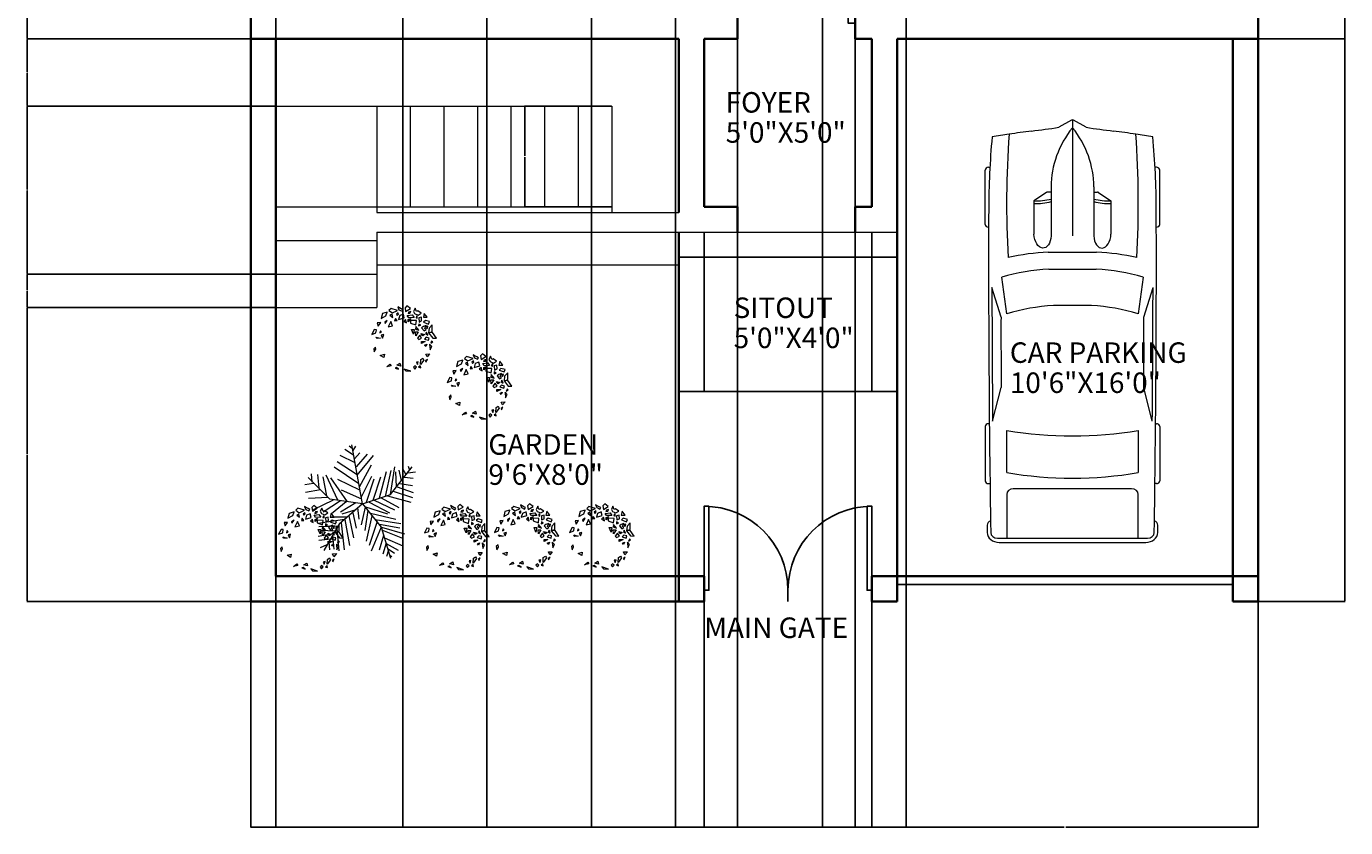
# Model space of a CAD drawing. Units: inches. Extents: x 25018 to 25490, y 41421 to 42101.
# Tile 1 of 5: x 25018 to 25490, y 41421 to 41707. Entities that reach past the tile are written whole.
import ezdxf

# ---------------------------------------------------------------- set-up
doc = ezdxf.new("R2010")
doc.units = ezdxf.units.IN
for name, color, linetype, lineweight in [('A-ANNO-DIMS', 2, 'Continuous', 18), ('A-ANNO-TEXT', 7, 'Continuous', 18), ('A-AREA-IDEN', 7, 'Continuous', 18), ('A-DOOR', 3, 'Continuous', 25), ('A-FLOR', 7, 'Continuous', 25), ('A-FLOR-STRS', 7, 'Continuous', 18), ('A-SITE-VEHI', 8, 'Continuous', 13), ('A-WALL', 7, 'Continuous', 35), ('L-PLNT-TREE', 94, 'Continuous', 13)]:
    doc.layers.add(name, color=color, linetype=linetype, lineweight=lineweight)
doc.styles.get("Standard").update_dxf_attribs({"font": 'arial.ttf'})
doc.dimstyles.get("Standard").update_dxf_attribs({"dimtxt": 0.18, "dimasz": 0.18, "dimexe": 0.18, "dimexo": 0.0625, "dimgap": 0.09, "dimtad": 0, "dimtih": 1, "dimtoh": 1, "dimdec": 4, "dimzin": 0, "dimdsep": 46, "dimtxsty": 'Standard', "dimcen": 0.09, "dimadec": 0, "dimazin": 0, "dimtfac": 1, "dimtdec": 4, "dimtofl": 0, "dimtmove": 0, "dimatfit": 3, "dimfxl": 1, "dimtolj": 1, "dimtzin": 0, "dimarcsym": 0})

# ---------------------------------------------------------------- blocks, each defined once
blk = doc.blocks.new('*U2')
for p, q in [((0, 0), (0, -100)), ((750, 0), (750, -100))]:
    blk.add_line(p, q)
blk.add_lwpolyline([(0, 0), (0, 750), (43.75, 750), (43.75, 0)], close=True)
blk.add_arc((0, 0), 750, 0, 90)
blk = doc.blocks.new('*U9')
for p, q in [((21.1, 37.41), (21.1, 36.83)), ((46.55, 38.89), (22.35, 38.89)), ((47.8, 37.39), (47.8, 37.41)), ((87.99, 31.87), (74.76, 35.92)), ((134.31, 35.6), (119.29, 31.78)), ((135.45, 37.07), (135.45, 37.41)), ((136.7, 38.89), (160.9, 38.89)), ((162.15, 37.41), (162.15, 36.77)), ((70.03, 31.54), (86.41, 29.35)), ((186.47, -33.5), (186.47, 33.5)), ((188.4, -32.76), (188.4, 32.76)), ((138.42, 29.35), (157.25, 29.35)), ((164.52, 26.39), (164.52, -26.39)), ((186.47, 29.35), (167.01, 29.35)), ((32.27, 11.63), (36.13, 17.17)), ((36.13, 17.17), (50.94, 17.17)), ((3.27, 6.13), (0.1, 0.41)), ((29.77, 9.51), (51.68, 9.51)), ((32.12, 9.51), (32.12, 11.15)), ((58.92, -10.77), (58.92, 10.77)), ((66.55, -10.53), (66.55, 10.53)), ((82.74, 8.5), (82.74, -8.5)), ((186.47, -10.53), (186.47, 10.53)), ((0, 0), (51.68, 0)), ((0.1, -0.41), (3.27, -6.13)), ((29.77, -9.51), (51.68, -9.51)), ((32.12, -9.51), (32.12, -11.15)), ((32.27, -11.63), (36.13, -17.17)), ((36.13, -17.17), (50.94, -17.17)), ((86.41, -29.35), (70.03, -31.54)), ((157.25, -29.35), (138.42, -29.35)), ((167.01, -29.35), (186.47, -29.35)), ((87.99, -31.87), (74.76, -35.92)), ((134.31, -35.6), (119.29, -31.78)), ((21.1, -37.41), (21.1, -36.83)), ((46.55, -38.89), (22.35, -38.89)), ((47.8, -37.39), (47.8, -37.41)), ((135.45, -37.07), (135.45, -37.41)), ((136.7, -38.89), (160.9, -38.89)), ((162.15, -37.41), (162.15, -36.77))]:
    blk.add_line(p, q)
for centre, major_axis, ratio, start_param, end_param in [((266.03, -27.52), (0, 313.31), 0.842304, 1.367076, 1.39176), ((41.19, -490.86), (0, 528.23), 0.842304, 0.00281, 0.075598), ((22.35, 37.41), (0, -1.48), 0.842304, 3.141593, 4.712389), ((64.48, -10555.62), (0, 10593.03), 0.842304, -0.013397, 0.002797), ((46.55, 37.41), (0, 1.48), 0.842304, -1.570796, 0), ((64.48, -10555.62), (0, -10591.55), 0.842304, 3.133765, 3.140441), ((136.7, 37.41), (0, -1.48), 0.842304, 3.141593, 4.712389), ((160.9, 37.41), (0, 1.48), 0.842304, -1.570796, 0), ((180.63, 35.84), (0, 2.22), 0.842304, -0.013017, 1.249894), ((64.48, -10556.36), (0, 10595.31), 0.842304, -0.013397, -0.013017), ((183.98, 33.5), (0, -2.96), 0.842304, 1.570796, 3.128196), ((183.98, 32.76), (0, -5.25), 0.842304, 1.570796, 3.128196), ((37.47, -593.96), (0, -623.33), 0.842304, 3.096046, 3.200911), ((135.29, 5.39), (0, 81.77), 0.842304, 1.245306, 1.50788), ((95.79, -3666.35), (0, -3698.24), 0.842304, 3.134049, 3.144098), ((259.18, -27.52), (0, -305.3), 0.842304, 4.528606, 4.561838), ((134.4, 5.39), (0, -89.78), 0.842304, 4.449482, 4.652344), ((149.6, 2.8), (0, -79.58), 0.842304, 4.372215, 4.640744), ((17.08, 0), (0, 147.02), 0.842304, 4.511394, 4.913384), ((35.91, 0), (0, 147.02), 0.842304, 4.511394, 4.913384), ((167.01, 26.39), (0, 2.96), 0.842304, 0, 1.570796), ((-204.49, 52.4), (0, -250.96), 0.842304, 1.385369, 1.434372), ((13.04, 17.01), (0, 27.42), 0.842304, 4.435146, 4.718221), ((14.2, 17.01), (0, 27.42), 0.842304, 4.435146, 4.718221), ((50.79, 13.34), (6.34, -0.36), 0.603834, -1.395552, 1.581315), ((29.77, -46.66), (0, 56.17), 0.842304, 0, 0.590319), ((32.75, 11.15), (0, 0.74), 0.842304, 0.879714, 1.570796), ((0.62, 0), (0, -0.74), 0.842304, 4.131459, 5.293319), ((29.77, 46.66), (0, 56.17), 0.842304, 2.551274, 3.141593), ((-204.49, -52.4), (0, 250.96), 0.842304, -1.434372, -1.385369), ((32.75, -11.15), (0, -0.74), 0.842304, 4.712389, 5.403472), ((13.04, -17.01), (0, -27.42), 0.842304, 1.564964, 1.848039), ((14.2, -17.01), (0, -27.42), 0.842304, 1.564964, 1.848039), ((134.4, -5.39), (0, -89.78), 0.842304, -1.510751, -1.307889), ((135.29, -5.39), (0, -81.77), 0.842304, -1.50788, -1.245306), ((149.6, -2.8), (0, -79.58), 0.842304, -1.499151, -1.230623), ((259.18, 27.52), (0, 305.3), 0.842304, 1.721348, 1.754579), ((266.03, 27.52), (0, 313.31), 0.842304, 1.749832, 1.774517), ((37.47, 593.96), (0, -623.33), 0.842304, -0.059319, 0.045547), ((167.01, -26.39), (0, -2.96), 0.842304, 4.712389, 6.283185), ((95.79, 3666.35), (0, -3698.24), 0.842304, -0.002505, 0.007544), ((183.98, -33.5), (0, 2.96), 0.842304, 3.15499, 4.712389), ((183.98, -32.76), (0, -5.25), 0.842304, 0.013397, 1.570796), ((41.19, 490.86), (0, -528.23), 0.842304, -0.075598, -0.00281), ((22.35, -37.41), (0, 1.48), 0.842304, 1.570796, 3.141593), ((64.48, 10555.62), (0, 10593.03), 0.842304, 3.138796, 3.15499), ((46.55, -37.41), (0, -1.48), 0.842304, 0, 1.570796), ((64.48, 10555.62), (0, -10591.55), 0.842304, 0.001152, 0.007828), ((136.7, -37.41), (0, -1.48), 0.842304, -1.570796, 0), ((160.9, -37.41), (0, 1.48), 0.842304, 3.141593, 4.712389), ((180.63, -35.84), (0, -2.22), 0.842304, -1.249894, 0.013017), ((64.48, 10556.36), (0, 10595.31), 0.842304, 3.15461, 3.15499)]:
    blk.add_ellipse(centre, major_axis=major_axis, ratio=ratio, start_param=start_param, end_param=end_param)
at = {"extrusion": (0, 0, -1)}
blk.add_ellipse((50.79, -13.34), major_axis=(6.34, 0.36), ratio=0.603834, start_param=-1.395552, end_param=1.581315, dxfattribs=at)
blk = doc.blocks.new('*U12')
for p, q in [((-8.737, 47.138), (-17.069, 52.711)), ((-10.186, 53.64), (-13.084, 55.962)), ((0, 0), (-10.5, 57)), ((-9.099, 51.782), (-6.563, 55.962)), ((-5.114, 28.097), (-24.676, 40.636)), ((-7.288, 39.707), (-21.778, 46.673)), ((-7.65, 43.423), (-2.578, 49.46)), ((-5.839, 35.992), (4.667, 48.067)), ((-5.114, 27.632), (10.463, 46.673)), ((-48.585, 21.131), (-49.309, 29.026)), ((-43.513, 28.561), (-42.427, 15.558)), ((-38.442, 26.239), (-34.819, 7.663)), ((-35.544, 28.097), (-24.314, 3.947)), ((-3.665, 19.273), (-27.574, 35.527)), ((-2.941, 16.486), (8.652, 37.85)), ((-1.129, 6.734), (9.014, 26.704)), ((10.101, 3.483), (17.708, 26.239)), ((16.259, 5.805), (23.142, 31.348)), ((22.055, 7.198), (27.489, 32.277)), ((27, 9), (48, 36)), ((27.127, 9.056), (31.112, 35.992)), ((31.836, 30.883), (32.561, 16.486)), ((35.096, 32.741), (37.27, 22.524)), ((38.719, 34.134), (41.979, 28.561)), ((40.53, 25.775), (48.862, 24.846)), ((43.791, 29.954), (51.036, 30.883)), ((44.153, 36.456), (45.239, 32.741)), ((-47.498, 19.737), (-55.83, 18.344)), ((-40.615, 13.7), (-55.105, 10.913)), ((-31.5, 4.5), (-52.5, 25.5)), ((-14.533, 2.09), (-30.834, 25.31)), ((-24.314, 23.917), (-2.941, 13.7)), ((-20.691, 13.7), (-1.129, 4.876)), ((3.942, 1.625), (11.187, 24.381)), ((33.285, 16.486), (48.862, 10.913)), ((36.183, 19.737), (48.137, 17.88)), ((-33.37, 6.269), (-52.207, 5.34)), ((-28.299, 3.483), (-47.86, -5.805)), ((-21.416, 3.018), (-38.079, -8.128)), ((0, 0), (-31.5, 4.5)), ((-15.982, 2.09), (-30.11, -9.521)), ((0, 0), (-22.5, -19.5)), ((-6.563, 1.161), (-21.416, -8.128)), ((0, 0), (27, 9)), ((0, 0), (18, -22.5)), ((6.478, 1.625), (26.04, -8.592)), ((11.187, 3.483), (30.749, -5.805)), ((18.07, 5.805), (35.096, -3.483)), ((24.229, 7.663), (46.688, 1.625)), ((29.662, 12.307), (48.137, 6.269)), ((-6.563, -5.805), (-19.967, -9.985)), ((-13.446, -11.378), (-8.737, -32.741)), ((-9.461, -8.592), (-6.201, -23.453)), ((-4.752, -3.483), (-3.665, -14.629)), ((2.493, -3.019), (-1.491, -20.202)), ((1.769, -2.555), (24.229, -9.521)), ((5.029, -6.27), (2.131, -25.775)), ((9.014, -11.378), (3.58, -35.992)), ((7.565, -9.056), (32.198, -14.629)), ((-17.431, -15.094), (-42.789, -18.809)), ((-24.314, -21.596), (-42.427, -22.06)), ((-22.5, -19.5), (-37.5, -45)), ((-15.257, -12.772), (-30.11, -12.772)), ((-25.038, -23.918), (-22.865, -45.281)), ((-20.691, -18.345), (-17.793, -44.352)), ((-17.069, -15.094), (-12.721, -40.172)), ((14.085, -16.951), (6.478, -40.172)), ((18.07, -22.524), (8.289, -45.745)), ((12.274, -15.094), (36.907, -18.809)), ((16.259, -19.738), (36.183, -22.989)), ((18, -22.5), (27, -52.5)), ((18.433, -22.524), (40.53, -29.026)), ((19.157, -25.311), (38.719, -33.206)), ((-28.299, -29.026), (-42.789, -31.348)), ((-30.834, -34.135), (-42.427, -35.528)), ((-26.849, -26.24), (-40.253, -25.775)), ((-32.646, -36.921), (-31.921, -44.352)), ((-29.023, -30.884), (-27.936, -43.887)), ((20.244, -30.419), (15.897, -44.816)), ((22.78, -37.85), (19.519, -48.532)), ((21.331, -32.741), (39.081, -40.636)), ((-34.457, -39.708), (-40.978, -42.494)), ((22.78, -38.314), (34.372, -44.816)), ((24.591, -45.745), (23.142, -50.854)), ((24.591, -43.423), (30.749, -47.603)), ((26.764, -49.925), (28.213, -50.854))]:
    blk.add_line(p, q)
blk = doc.blocks.new('*U13')
for points in [[(-5.78, 9.75), (-7.54, 9.23), (-8.01, 7.5), (-6.26, 8.45)], [(-4.43, 11.05), (-5.18, 10.36), (-3.96, 9.49), (-2.07, 10.36)], [(-1.94, 9.49), (-2.48, 8.97), (-2.27, 8.54), (-1.8, 9.06)], [(-2, 11.66), (-1.6, 10.62), (-0.52, 10.1), (-0.18, 10.62), (-0.79, 10.96)], [(1.24, 12), (0.56, 11.31), (0.76, 10.01), (2.52, 11.05)], [(2.59, 9.93), (1.84, 9.75), (1.64, 9.23), (2.32, 9.41)], [(4.14, 11.14), (3.6, 10.01), (4, 9.23), (5.22, 8.71), (6.3, 9.41), (5.08, 10.19), (4.61, 10.01)], [(-8.14, 6.03), (-9.36, 5.95), (-9.02, 4.73)], [(-5.78, 6.81), (-6.66, 6.21), (-6.52, 5.69)], [(-4.57, 6.38), (-5.45, 4.47), (-3.89, 4.82)], [(-4.84, 8.63), (-3.83, 7.85), (-4.03, 8.97)], [(-2.88, 7.5), (-3.15, 6.64), (-2.27, 6.72)], [(0.02, 9.06), (-1.33, 8.54), (-1.73, 7.16), (0.29, 7.76)], [(0.76, 7.16), (0.09, 6.46), (1.1, 5.95)], [(1.37, 8.54), (3.13, 8.8), (3.8, 7.85), (1.91, 7.76)], [(1.71, 6.29), (1.71, 7.07), (2.65, 7.5), (2.11, 6.9)], [(2.52, 6.81), (2.52, 5.86), (4.41, 5.17), (4.61, 6.72)], [(4.61, 8.28), (4.54, 7.76), (4.95, 7.59), (4.95, 8.28)], [(5.49, 5.51), (5.42, 4.82), (6.16, 5.08)], [(6.43, 7.94), (5.49, 7.68), (5.56, 6.21), (6.5, 6.64)], [(8.12, 4.99), (7.11, 4.65), (6.5, 4.13), (7.38, 3.09), (8.12, 3.52), (7.65, 3.87)], [(7.45, 9.32), (7.11, 7.94), (8.52, 7.94)], [(7.85, 6.81), (7.18, 6.21), (9, 5.51), (9.33, 6.38)], [(8.73, 4.73), (8.19, 4.56), (8.39, 3.87), (8.59, 4.04)], [(10.28, 5.17), (9.2, 4.04), (9, 2.31), (10.48, 0.49), (11.76, 0.41), (10.35, 2.48), (9.33, 2.4), (10.28, 2.83)], [(-11.32, 1.79), (-9.83, 2.31), (-9.63, 3.44), (-10.44, 3.52)], [(-8.21, 0.41), (-9.43, 0.32), (-9.83, 0.84)], [(-8.21, 3.09), (-8.48, 2.31), (-7.87, 2.57)], [(-7, 1.79), (-7.94, 1.53), (-7.47, 0.49)], [(3.53, 1.88), (2.86, 3.52), (3.8, 3.52)], [(4.41, 4.56), (4.27, 3.7), (5.49, 3.26)], [(4.27, 2.74), (5.29, 2.66), (4.41, 1.27)], [(5.83, 1.53), (5.02, 0.41), (5.49, -0.02), (6.5, 0.41)], [(7.51, 1.71), (6.91, 1.27), (6.23, 2.14)], [(8.12, 0.75), (7.51, 0.15), (8.93, -0.28), (9.13, 0.49)], [(8.19, 2.57), (7.92, 2.05), (8.66, 1.53)], [(-10.03, -2.71), (-10.64, -3.31), (-10.44, -4.44), (-9.9, -3.49)], [(7.78, -0.8), (6.43, -1.5), (6.43, -0.72)], [(8.32, -1.75), (7.98, -2.53), (7.58, -2.1)], [(9.33, -1.75), (9.54, -3.74), (10.14, -2.53)], [(10.08, -0.63), (9.74, -1.32), (10.48, -0.89)], [(-8.28, -5.73), (-6.79, -5.3), (-7, -6.51)], [(-4.84, -8.85), (-4.43, -9.45), (-5.99, -9.8)], [(-2.34, -9.2), (-1.26, -8.5), (-0.99, -9.54)], [(5.29, -7.98), (4.61, -8.16), (5.02, -8.94)], [(6.1, -8.94), (6.16, -7.21), (6.91, -6.69), (7.24, -7.38)], [(8.05, -8.07), (8.59, -7.12), (7.92, -7.55)], [(9.33, -5.13), (8.46, -6.25), (7.98, -5.22)], [(-2.54, -10.06), (-3.02, -10.23), (-1.8, -10.67)], [(0.22, -10.58), (0.83, -11.27), (2.59, -11.36)], [(4.07, -9.45), (3.53, -9.97), (4.07, -10.58), (4.61, -9.89)], [(6.03, -9.45), (5.42, -9.97), (6.16, -10.15)]]:
    blk.add_lwpolyline(points, close=True)
blk = doc.blocks.new('*D39')
at = {"layer": 'A-ANNO-DIMS', "color": 0, "lineweight": -2, "transparency": 16777216}
for p, q in [((25458.72, 42070.05), (25489.83, 42070.05)), ((25489.65, 42069.87), (25489.65, 41785.98)), ((25489.65, 41501.73), (25489.65, 41785.62)), ((25458.72, 41501.55), (25489.83, 41501.55))]:
    blk.add_line(p, q, dxfattribs=at)
at = {"layer": 'A-ANNO-DIMS', "color": 0, "transparency": 16777216}
for points in [[(25489.62, 42069.87), (25489.68, 42069.87), (25489.65, 42070.05)], [(25489.62, 41501.73), (25489.68, 41501.73), (25489.65, 41501.55)]]:
    blk.add_solid(points, dxfattribs=at)
at = {"layer": 'Defpoints', "color": 0, "transparency": 16777216}
for p in [(25458.65, 42070.05), (25489.65, 42070.05), (25458.65, 41501.55)]:
    blk.add_point(p, dxfattribs=at)
at = {"layer": 'A-ANNO-DIMS', "color": 0, "transparency": 16777216, "insert": (25489.65, 41785.8), "char_height": 0.18, "attachment_point": 5}
blk.add_mtext('\\A1;568.5', dxfattribs=at)
blk = doc.blocks.new('*D40')
at = {"layer": 'A-ANNO-DIMS', "color": 0, "lineweight": -2, "transparency": 16777216}
for p, q in [((25107.59, 41606.55), (25018.58, 41606.55)), ((25018.76, 41606.37), (25018.76, 41554.23)), ((25018.76, 41501.73), (25018.76, 41553.87)), ((25098.59, 41501.55), (25018.58, 41501.55))]:
    blk.add_line(p, q, dxfattribs=at)
at = {"layer": 'A-ANNO-DIMS', "color": 0, "transparency": 16777216}
for points in [[(25018.73, 41606.37), (25018.79, 41606.37), (25018.76, 41606.55)], [(25018.73, 41501.73), (25018.79, 41501.73), (25018.76, 41501.55)]]:
    blk.add_solid(points, dxfattribs=at)
at = {"layer": 'Defpoints', "color": 0, "transparency": 16777216}
for p in [(25018.76, 41606.55), (25107.65, 41606.55), (25098.65, 41501.55)]:
    blk.add_point(p, dxfattribs=at)
at = {"layer": 'A-ANNO-DIMS', "color": 0, "transparency": 16777216, "insert": (25018.76, 41554.05), "char_height": 0.18, "attachment_point": 5}
blk.add_mtext('\\A1;105', dxfattribs=at)
blk = doc.blocks.new('*D41')
at = {"layer": 'A-ANNO-DIMS', "color": 0, "lineweight": -2, "transparency": 16777216}
for p, q in [((25107.59, 41618.55), (25018.58, 41618.55)), ((25018.76, 41618.37), (25018.76, 41612.73)), ((25018.76, 41606.73), (25018.76, 41612.37)), ((25107.59, 41606.55), (25018.58, 41606.55))]:
    blk.add_line(p, q, dxfattribs=at)
at = {"layer": 'A-ANNO-DIMS', "color": 0, "transparency": 16777216}
for points in [[(25018.73, 41618.37), (25018.79, 41618.37), (25018.76, 41618.55)], [(25018.73, 41606.73), (25018.79, 41606.73), (25018.76, 41606.55)]]:
    blk.add_solid(points, dxfattribs=at)
at = {"layer": 'Defpoints', "color": 0, "transparency": 16777216}
for p in [(25018.76, 41618.55), (25107.65, 41618.55), (25107.65, 41606.55)]:
    blk.add_point(p, dxfattribs=at)
at = {"layer": 'A-ANNO-DIMS', "color": 0, "transparency": 16777216, "insert": (25018.76, 41612.55), "char_height": 0.18, "attachment_point": 5}
blk.add_mtext('\\A1;12', dxfattribs=at)
blk = doc.blocks.new('*D42')
at = {"layer": 'A-ANNO-DIMS', "color": 0, "lineweight": -2, "transparency": 16777216}
for p, q in [((25107.59, 41678.55), (25018.58, 41678.55)), ((25018.76, 41678.37), (25018.76, 41648.73)), ((25018.76, 41618.73), (25018.76, 41648.37)), ((25107.59, 41618.55), (25018.58, 41618.55))]:
    blk.add_line(p, q, dxfattribs=at)
at = {"layer": 'A-ANNO-DIMS', "color": 0, "transparency": 16777216}
for points in [[(25018.73, 41678.37), (25018.79, 41678.37), (25018.76, 41678.55)], [(25018.73, 41618.73), (25018.79, 41618.73), (25018.76, 41618.55)]]:
    blk.add_solid(points, dxfattribs=at)
at = {"layer": 'Defpoints', "color": 0, "transparency": 16777216}
for p in [(25018.76, 41678.55), (25107.65, 41678.55), (25107.65, 41618.55)]:
    blk.add_point(p, dxfattribs=at)
at = {"layer": 'A-ANNO-DIMS', "color": 0, "transparency": 16777216, "insert": (25018.76, 41648.55), "char_height": 0.18, "attachment_point": 5}
blk.add_mtext('\\A1;60', dxfattribs=at)
blk = doc.blocks.new('*D43')
at = {"layer": 'A-ANNO-DIMS', "color": 0, "lineweight": -2, "transparency": 16777216}
for p, q in [((25098.59, 41702.55), (25018.58, 41702.55)), ((25018.76, 41702.37), (25018.76, 41690.73)), ((25018.76, 41678.73), (25018.76, 41690.37)), ((25107.59, 41678.55), (25018.58, 41678.55))]:
    blk.add_line(p, q, dxfattribs=at)
at = {"layer": 'A-ANNO-DIMS', "color": 0, "transparency": 16777216}
for points in [[(25018.73, 41702.37), (25018.79, 41702.37), (25018.76, 41702.55)], [(25018.73, 41678.73), (25018.79, 41678.73), (25018.76, 41678.55)]]:
    blk.add_solid(points, dxfattribs=at)
at = {"layer": 'Defpoints', "color": 0, "transparency": 16777216}
for p in [(25018.76, 41702.55), (25098.65, 41702.55), (25107.65, 41678.55)]:
    blk.add_point(p, dxfattribs=at)
at = {"layer": 'A-ANNO-DIMS', "color": 0, "transparency": 16777216, "insert": (25018.76, 41690.55), "char_height": 0.18, "attachment_point": 5}
blk.add_mtext('\\A1;24', dxfattribs=at)
blk = doc.blocks.new('*D44')
at = {"layer": 'A-ANNO-DIMS', "color": 0, "lineweight": -2, "transparency": 16777216}
for p, q in [((25098.59, 41731.2), (25018.58, 41731.2)), ((25018.76, 41731.02), (25018.76, 41717.06)), ((25018.76, 41702.73), (25018.76, 41716.69)), ((25098.59, 41702.55), (25018.58, 41702.55))]:
    blk.add_line(p, q, dxfattribs=at)
at = {"layer": 'A-ANNO-DIMS', "color": 0, "transparency": 16777216}
for points in [[(25018.73, 41731.02), (25018.79, 41731.02), (25018.76, 41731.2)], [(25018.73, 41702.73), (25018.79, 41702.73), (25018.76, 41702.55)]]:
    blk.add_solid(points, dxfattribs=at)
at = {"layer": 'Defpoints', "color": 0, "transparency": 16777216}
for p in [(25018.76, 41731.2), (25098.65, 41731.2), (25098.65, 41702.55)]:
    blk.add_point(p, dxfattribs=at)
at = {"layer": 'A-ANNO-DIMS', "color": 0, "transparency": 16777216, "insert": (25018.76, 41716.88), "char_height": 0.18, "attachment_point": 5}
blk.add_mtext('\\A1;28.65', dxfattribs=at)
blk = doc.blocks.new('*D50')
at = {"layer": 'A-ANNO-DIMS', "color": 0, "lineweight": -2, "transparency": 16777216}
for p, q in [((25098.65, 41501.49), (25098.65, 41420.7)), ((25260.65, 41501.49), (25260.65, 41420.7)), ((25098.83, 41420.88), (25179.37, 41420.88)), ((25260.47, 41420.88), (25179.93, 41420.88))]:
    blk.add_line(p, q, dxfattribs=at)
at = {"layer": 'A-ANNO-DIMS', "color": 0, "transparency": 16777216}
for points in [[(25098.83, 41420.91), (25098.83, 41420.85), (25098.65, 41420.88)], [(25260.47, 41420.91), (25260.47, 41420.85), (25260.65, 41420.88)]]:
    blk.add_solid(points, dxfattribs=at)
at = {"layer": 'Defpoints', "color": 0, "transparency": 16777216}
for p in [(25098.65, 41501.55), (25260.65, 41501.55), (25260.65, 41420.88)]:
    blk.add_point(p, dxfattribs=at)
at = {"layer": 'A-ANNO-DIMS', "color": 0, "transparency": 16777216, "insert": (25179.65, 41420.88), "char_height": 0.18, "attachment_point": 5}
blk.add_mtext('\\A1;162', dxfattribs=at)
blk = doc.blocks.new('*D51')
at = {"layer": 'A-ANNO-DIMS', "color": 0, "lineweight": -2, "transparency": 16777216}
for p, q in [((25260.65, 41501.49), (25260.65, 41420.7)), ((25320.65, 41501.49), (25320.65, 41420.7)), ((25260.83, 41420.88), (25290.43, 41420.88)), ((25320.47, 41420.88), (25290.87, 41420.88))]:
    blk.add_line(p, q, dxfattribs=at)
at = {"layer": 'A-ANNO-DIMS', "color": 0, "transparency": 16777216}
for points in [[(25260.83, 41420.91), (25260.83, 41420.85), (25260.65, 41420.88)], [(25320.47, 41420.91), (25320.47, 41420.85), (25320.65, 41420.88)]]:
    blk.add_solid(points, dxfattribs=at)
at = {"layer": 'Defpoints', "color": 0, "transparency": 16777216}
for p in [(25260.65, 41501.55), (25320.65, 41501.55), (25320.65, 41420.88)]:
    blk.add_point(p, dxfattribs=at)
at = {"layer": 'A-ANNO-DIMS', "color": 0, "transparency": 16777216, "insert": (25290.65, 41420.88), "char_height": 0.18, "attachment_point": 5}
blk.add_mtext('\\A1;60', dxfattribs=at)
blk = doc.blocks.new('*D52')
at = {"layer": 'A-ANNO-DIMS', "color": 0, "lineweight": -2, "transparency": 16777216}
for p, q in [((25320.65, 41501.49), (25320.65, 41420.7)), ((25458.65, 41501.49), (25458.65, 41420.7)), ((25320.83, 41420.88), (25389.37, 41420.88)), ((25458.47, 41420.88), (25389.93, 41420.88))]:
    blk.add_line(p, q, dxfattribs=at)
at = {"layer": 'A-ANNO-DIMS', "color": 0, "transparency": 16777216}
for points in [[(25320.83, 41420.91), (25320.83, 41420.85), (25320.65, 41420.88)], [(25458.47, 41420.91), (25458.47, 41420.85), (25458.65, 41420.88)]]:
    blk.add_solid(points, dxfattribs=at)
at = {"layer": 'Defpoints', "color": 0, "transparency": 16777216}
for p in [(25320.65, 41501.55), (25458.65, 41501.55), (25458.65, 41420.88)]:
    blk.add_point(p, dxfattribs=at)
at = {"layer": 'A-ANNO-DIMS', "color": 0, "transparency": 16777216, "insert": (25389.65, 41420.88), "char_height": 0.18, "attachment_point": 5}
blk.add_mtext('\\A1;138', dxfattribs=at)
blk = doc.blocks.new('*D53')
at = {"layer": 'A-ANNO-DIMS', "color": 0, "lineweight": -2, "transparency": 16777216}
for p, q in [((25272.65, 41702.49), (25272.65, 41420.7)), ((25314.65, 41702.49), (25314.65, 41420.7)), ((25272.83, 41420.88), (25293.43, 41420.88)), ((25314.47, 41420.88), (25293.87, 41420.88))]:
    blk.add_line(p, q, dxfattribs=at)
at = {"layer": 'A-ANNO-DIMS', "color": 0, "transparency": 16777216}
for points in [[(25272.83, 41420.91), (25272.83, 41420.85), (25272.65, 41420.88)], [(25314.47, 41420.91), (25314.47, 41420.85), (25314.65, 41420.88)]]:
    blk.add_solid(points, dxfattribs=at)
at = {"layer": 'Defpoints', "color": 0, "transparency": 16777216}
for p in [(25272.65, 41702.55), (25314.65, 41702.55), (25314.65, 41420.88)]:
    blk.add_point(p, dxfattribs=at)
at = {"layer": 'A-ANNO-DIMS', "color": 0, "transparency": 16777216, "insert": (25293.65, 41420.88), "char_height": 0.18, "attachment_point": 5}
blk.add_mtext('\\A1;42', dxfattribs=at)
blk = doc.blocks.new('*D54')
at = {"layer": 'A-ANNO-DIMS', "color": 0, "lineweight": -2, "transparency": 16777216}
for p, q in [((25458.72, 41756.26), (25489.83, 41756.26)), ((25489.65, 41756.08), (25489.65, 41729.59)), ((25489.65, 41702.73), (25489.65, 41729.22)), ((25458.72, 41702.55), (25489.83, 41702.55))]:
    blk.add_line(p, q, dxfattribs=at)
at = {"layer": 'A-ANNO-DIMS', "color": 0, "transparency": 16777216}
for points in [[(25489.62, 41756.08), (25489.68, 41756.08), (25489.65, 41756.26)], [(25489.62, 41702.73), (25489.68, 41702.73), (25489.65, 41702.55)]]:
    blk.add_solid(points, dxfattribs=at)
at = {"layer": 'Defpoints', "color": 0, "transparency": 16777216}
for p in [(25458.65, 41756.26), (25489.65, 41756.26), (25458.65, 41702.55)]:
    blk.add_point(p, dxfattribs=at)
at = {"layer": 'A-ANNO-DIMS', "color": 0, "transparency": 16777216, "insert": (25489.65, 41729.4), "char_height": 0.18, "attachment_point": 5}
blk.add_mtext('\\A1;53.71', dxfattribs=at)
blk = doc.blocks.new('*D66')
at = {"layer": 'A-ANNO-DIMS', "color": 0, "lineweight": -2, "transparency": 16777216}
for p, q in [((25107.65, 41903.49), (25107.65, 41420.7)), ((25152.99, 41903.49), (25152.99, 41420.7)), ((25107.83, 41420.88), (25129.92, 41420.88)), ((25152.81, 41420.88), (25130.72, 41420.88))]:
    blk.add_line(p, q, dxfattribs=at)
at = {"layer": 'A-ANNO-DIMS', "color": 0, "transparency": 16777216}
for points in [[(25107.83, 41420.91), (25107.83, 41420.85), (25107.65, 41420.88)], [(25152.81, 41420.91), (25152.81, 41420.85), (25152.99, 41420.88)]]:
    blk.add_solid(points, dxfattribs=at)
at = {"layer": 'Defpoints', "color": 0, "transparency": 16777216}
for p in [(25107.65, 41903.55), (25152.99, 41903.55), (25152.99, 41420.88)]:
    blk.add_point(p, dxfattribs=at)
at = {"layer": 'A-ANNO-DIMS', "color": 0, "transparency": 16777216, "insert": (25130.32, 41420.88), "char_height": 0.18, "attachment_point": 5}
blk.add_mtext('\\A1;45.34', dxfattribs=at)
blk = doc.blocks.new('*D67')
at = {"layer": 'A-ANNO-DIMS', "color": 0, "lineweight": -2, "transparency": 16777216}
for p, q in [((25152.99, 41903.49), (25152.99, 41420.7)), ((25182.99, 41903.49), (25182.99, 41420.7)), ((25153.17, 41420.88), (25167.77, 41420.88)), ((25182.81, 41420.88), (25168.21, 41420.88))]:
    blk.add_line(p, q, dxfattribs=at)
at = {"layer": 'A-ANNO-DIMS', "color": 0, "transparency": 16777216}
for points in [[(25153.17, 41420.91), (25153.17, 41420.85), (25152.99, 41420.88)], [(25182.81, 41420.91), (25182.81, 41420.85), (25182.99, 41420.88)]]:
    blk.add_solid(points, dxfattribs=at)
at = {"layer": 'Defpoints', "color": 0, "transparency": 16777216}
for p in [(25152.99, 41903.55), (25182.99, 41903.55), (25182.99, 41420.88)]:
    blk.add_point(p, dxfattribs=at)
at = {"layer": 'A-ANNO-DIMS', "color": 0, "transparency": 16777216, "insert": (25167.99, 41420.88), "char_height": 0.18, "attachment_point": 5}
blk.add_mtext('\\A1;30', dxfattribs=at)
blk = doc.blocks.new('*D68')
at = {"layer": 'A-ANNO-DIMS', "color": 0, "lineweight": -2, "transparency": 16777216}
for p, q in [((25182.99, 41903.49), (25182.99, 41420.7)), ((25220.45, 41903.49), (25220.45, 41420.7)), ((25183.17, 41420.88), (25201.26, 41420.88)), ((25220.27, 41420.88), (25202.18, 41420.88))]:
    blk.add_line(p, q, dxfattribs=at)
at = {"layer": 'A-ANNO-DIMS', "color": 0, "transparency": 16777216}
for points in [[(25183.17, 41420.91), (25183.17, 41420.85), (25182.99, 41420.88)], [(25220.27, 41420.91), (25220.27, 41420.85), (25220.45, 41420.88)]]:
    blk.add_solid(points, dxfattribs=at)
at = {"layer": 'Defpoints', "color": 0, "transparency": 16777216}
for p in [(25182.99, 41903.55), (25220.45, 41903.55), (25220.45, 41420.88)]:
    blk.add_point(p, dxfattribs=at)
at = {"layer": 'A-ANNO-DIMS', "color": 0, "transparency": 16777216, "insert": (25201.72, 41420.88), "char_height": 0.18, "attachment_point": 5}
blk.add_mtext('\\A1;37.464', dxfattribs=at)
blk = doc.blocks.new('*D69')
at = {"layer": 'A-ANNO-DIMS', "color": 0, "lineweight": -2, "transparency": 16777216}
for p, q in [((25220.45, 41903.49), (25220.45, 41420.7)), ((25250.45, 41903.49), (25250.45, 41420.7)), ((25220.63, 41420.88), (25235.23, 41420.88)), ((25250.27, 41420.88), (25235.67, 41420.88))]:
    blk.add_line(p, q, dxfattribs=at)
at = {"layer": 'A-ANNO-DIMS', "color": 0, "transparency": 16777216}
for points in [[(25220.63, 41420.91), (25220.63, 41420.85), (25220.45, 41420.88)], [(25250.27, 41420.91), (25250.27, 41420.85), (25250.45, 41420.88)]]:
    blk.add_solid(points, dxfattribs=at)
at = {"layer": 'Defpoints', "color": 0, "transparency": 16777216}
for p in [(25220.45, 41903.55), (25250.45, 41903.55), (25250.45, 41420.88)]:
    blk.add_point(p, dxfattribs=at)
at = {"layer": 'A-ANNO-DIMS', "color": 0, "transparency": 16777216, "insert": (25235.45, 41420.88), "char_height": 0.18, "attachment_point": 5}
blk.add_mtext('\\A1;30', dxfattribs=at)
blk = doc.blocks.new('*D70')
at = {"layer": 'A-ANNO-DIMS', "color": 0, "lineweight": -2, "transparency": 16777216}
for p, q in [((25250.45, 41903.49), (25250.45, 41420.7)), ((25302.95, 41903.49), (25302.95, 41420.7)), ((25250.63, 41420.88), (25276.38, 41420.88)), ((25302.77, 41420.88), (25277.03, 41420.88))]:
    blk.add_line(p, q, dxfattribs=at)
at = {"layer": 'A-ANNO-DIMS', "color": 0, "transparency": 16777216}
for points in [[(25250.63, 41420.91), (25250.63, 41420.85), (25250.45, 41420.88)], [(25302.77, 41420.91), (25302.77, 41420.85), (25302.95, 41420.88)]]:
    blk.add_solid(points, dxfattribs=at)
at = {"layer": 'Defpoints', "color": 0, "transparency": 16777216}
for p in [(25250.45, 41903.55), (25302.95, 41903.55), (25302.95, 41420.88)]:
    blk.add_point(p, dxfattribs=at)
at = {"layer": 'A-ANNO-DIMS', "color": 0, "transparency": 16777216, "insert": (25276.7, 41420.88), "char_height": 0.18, "attachment_point": 5}
blk.add_mtext('\\A1;52.5', dxfattribs=at)
blk = doc.blocks.new('*D71')
at = {"layer": 'A-ANNO-DIMS', "color": 0, "lineweight": -2, "transparency": 16777216}
for p, q in [((25302.95, 41903.49), (25302.95, 41420.7)), ((25332.95, 41903.49), (25332.95, 41420.7)), ((25303.13, 41420.88), (25317.73, 41420.88)), ((25332.77, 41420.88), (25318.17, 41420.88))]:
    blk.add_line(p, q, dxfattribs=at)
at = {"layer": 'A-ANNO-DIMS', "color": 0, "transparency": 16777216}
for points in [[(25303.13, 41420.91), (25303.13, 41420.85), (25302.95, 41420.88)], [(25332.77, 41420.91), (25332.77, 41420.85), (25332.95, 41420.88)]]:
    blk.add_solid(points, dxfattribs=at)
at = {"layer": 'Defpoints', "color": 0, "transparency": 16777216}
for p in [(25302.95, 41903.55), (25332.95, 41903.55), (25332.95, 41420.88)]:
    blk.add_point(p, dxfattribs=at)
at = {"layer": 'A-ANNO-DIMS', "color": 0, "transparency": 16777216, "insert": (25317.95, 41420.88), "char_height": 0.18, "attachment_point": 5}
blk.add_mtext('\\A1;30', dxfattribs=at)
blk = doc.blocks.new('*D74')
at = {"layer": 'A-ANNO-DIMS', "color": 0, "lineweight": -2, "transparency": 16777216}
for p, q in [((25227.59, 41678.55), (25196.47, 41678.55)), ((25196.65, 41678.37), (25196.65, 41660.73)), ((25196.65, 41642.73), (25196.65, 41660.37)), ((25227.59, 41642.55), (25196.47, 41642.55))]:
    blk.add_line(p, q, dxfattribs=at)
at = {"layer": 'A-ANNO-DIMS', "color": 0, "transparency": 16777216}
for points in [[(25196.62, 41678.37), (25196.68, 41678.37), (25196.65, 41678.55)], [(25196.62, 41642.73), (25196.68, 41642.73), (25196.65, 41642.55)]]:
    blk.add_solid(points, dxfattribs=at)
at = {"layer": 'Defpoints', "color": 0, "transparency": 16777216}
for p in [(25196.65, 41678.55), (25227.65, 41678.55), (25227.65, 41642.55)]:
    blk.add_point(p, dxfattribs=at)
at = {"layer": 'A-ANNO-DIMS', "color": 0, "transparency": 16777216, "insert": (25196.65, 41660.55), "char_height": 0.18, "attachment_point": 5}
blk.add_mtext('\\A1;36', dxfattribs=at)

msp = doc.modelspace()

# ---------------------------------------------------------------- linework, layer by layer
at = {"layer": 'A-DOOR'}
msp.add_line((25329.6526, 41507.5498), (25449.6526, 41507.5498), dxfattribs=at)
at = {"layer": 'A-FLOR'}
for p, q in [((25260.6526, 41633.5498), (25260.6526, 41576.5498)), ((25320.6526, 41633.5498), (25320.6526, 41576.5498)), ((25251.6526, 41624.5498), (25329.6526, 41624.5498)), ((25251.6526, 41576.5498), (25329.6526, 41576.5498))]:
    msp.add_line(p, q, dxfattribs=at)
at = {"layer": 'A-FLOR-STRS'}
for p, q in [((25107.6526, 41678.5498), (25227.6526, 41678.5498)), ((25143.6526, 41678.5498), (25143.6526, 41640.5498)), ((25155.6526, 41678.5498), (25155.6526, 41642.5498)), ((25167.6526, 41678.5498), (25167.6526, 41642.5498)), ((25179.6526, 41678.5498), (25179.6526, 41642.5498)), ((25191.6526, 41678.5498), (25191.6526, 41642.5498)), ((25203.6526, 41678.5498), (25203.6526, 41642.5498)), ((25215.6526, 41678.5498), (25215.6526, 41642.5498)), ((25227.6526, 41678.5498), (25227.6526, 41640.5498)), ((25107.6526, 41642.5498), (25227.6526, 41642.5498)), ((25143.6526, 41640.5498), (25251.6526, 41640.5498)), ((25107.6526, 41630.5498), (25143.6526, 41630.5498)), ((25143.6526, 41633.5498), (25143.6526, 41606.5498)), ((25143.6526, 41633.5498), (25329.6526, 41633.5498)), ((25143.6526, 41621.7876), (25251.6526, 41621.7876)), ((25107.6526, 41618.5498), (25143.6526, 41618.5498)), ((25107.6526, 41606.5498), (25143.6526, 41606.5498))]:
    msp.add_line(p, q, dxfattribs=at)
at = {"layer": 'A-WALL'}
for p, q in [((25098.6526, 42070.0498), (25098.6526, 41501.5498)), ((25458.6526, 42070.0498), (25458.6526, 41501.5498)), ((25272.6526, 41702.5498), (25272.6526, 41711.5498)), ((25314.6526, 41702.5498), (25314.6526, 41711.5498)), ((25098.6526, 41702.5498), (25251.6526, 41702.5498)), ((25107.6526, 41702.5498), (25107.6526, 41510.5498)), ((25251.6526, 41702.5498), (25251.6526, 41640.5498)), ((25260.6526, 41702.5498), (25260.6526, 41642.5498)), ((25260.6526, 41702.5498), (25272.6526, 41702.5498)), ((25314.6526, 41702.5498), (25320.6526, 41702.5498)), ((25320.6526, 41702.5498), (25320.6526, 41642.5498)), ((25329.6526, 41702.5498), (25329.6526, 41501.5498)), ((25329.6526, 41702.5498), (25458.6526, 41702.5498)), ((25449.6526, 41702.5498), (25449.6526, 41501.5498)), ((25260.6526, 41642.5498), (25272.6526, 41642.5498)), ((25272.6526, 41633.5498), (25272.6526, 41642.5498)), ((25314.6526, 41633.5498), (25314.6526, 41642.5498)), ((25314.6526, 41642.5498), (25320.6526, 41642.5498)), ((25251.6526, 41633.5498), (25251.6526, 41501.5498)), ((25107.6526, 41510.5498), (25260.6526, 41510.5498)), ((25251.6526, 41510.5498), (25251.6526, 41501.5498)), ((25260.6526, 41510.5498), (25260.6526, 41501.5498)), ((25260.6526, 41510.5498), (25260.6526, 41501.5498)), ((25320.6526, 41510.5498), (25320.6526, 41501.5498)), ((25320.6526, 41510.5498), (25458.6526, 41510.5498)), ((25098.6526, 41501.5498), (25260.6526, 41501.5498)), ((25320.6526, 41501.5498), (25329.6526, 41501.5498)), ((25449.6526, 41501.5498), (25458.6526, 41501.5498))]:
    msp.add_line(p, q, dxfattribs=at)

# ---------------------------------------------------------------- block references
at = {"layer": 'A-DOOR'}
for p, xscale, yscale, zscale in [((25314.6526, 41708.1498), -0.0560000000000015, 0.0560000000000015, 0.0560000000000015), ((25260.6526, 41505.5498), 0.0400000000000011, 0.0400000000000011, 0.0400000000000011), ((25320.6526, 41505.5498), -0.0400000000000011, 0.0400000000000011, 0.0400000000000011)]:
    msp.add_blockref('*U2', p, dxfattribs=dict(at, xscale=xscale, yscale=yscale, zscale=zscale))
at = {"layer": 'A-SITE-VEHI', "xscale": 0.801346155695646, "yscale": 0.801346155695646, "zscale": 0.801346155695646, "rotation": 270}
msp.add_blockref('*U9', (25392.3368, 41673.5985), dxfattribs=at)
at = {"layer": 'L-PLNT-TREE'}
for p in [(25153.2206, 41595.1746), (25180.1927, 41578.0266), (25119.9028, 41523.7705), (25172.0707, 41524.2045), (25197.0519, 41524.4399), (25223.9184, 41524.4399)]:
    msp.add_blockref('*U13', p, dxfattribs=at)
at = {"layer": 'L-PLNT-TREE', "xscale": 0.3696653194007371, "yscale": 0.3696653194007371, "zscale": 0.3696653194007371}
msp.add_blockref('*U12', (25138.6084, 41536.3888), dxfattribs=at)

# ---------------------------------------------------------------- texts
at = {"layer": 'A-ANNO-TEXT'}
msp.add_text('MAIN GATE', height=7.32047, dxfattribs=at).set_placement((25260.7527, 41488.4709))
at = {"layer": 'A-AREA-IDEN'}
for s, height, p in [('FOYER', 7.32047, (25268.3819, 41676.2366)), ('5\'0"X5\'0"', 7.32047, (25268.3895, 41665.4773)), ('SITOUT', 7.32047, (25271.2283, 41602.8322)), ('5\'0"X4\'0"', 7.32047, (25271.2359, 41592.073)), ('CAR PARKING', 7.320471, (25369.9479, 41586.8007)), ('10\'6"X16\'0"', 7.320471, (25369.9555, 41576.0414)), ('GARDEN', 7.32047, (25183.5673, 41553.9673)), ('9\'6\'X8\'0"', 7.32047, (25183.5749, 41543.208))]:
    msp.add_text(s, height=height, dxfattribs=at).set_placement(p)

# ---------------------------------------------------------------- dimensions: what is measured, and where the dimension line sits
at = {"layer": 'A-ANNO-DIMS'}
for base, p1, p2, override, picture, middle in [((25489.6526, 42070.0498), (25458.6526, 41501.5498), (25458.6526, 42070.0498), {"dimdec": 1, "dimlfac": 1, "dimrnd": 0, "dimzin": 0, "dimdsep": 46, "dimlunit": 2}, '*D39', (25489.6526, 41785.7998)), ((25489.6526, 41756.2579), (25458.6526, 41702.5498), (25458.6526, 41756.2579), {"dimdec": 2, "dimlfac": 1, "dimrnd": 0, "dimzin": 0, "dimdsep": 46, "dimlunit": 2}, '*D54', (25489.6526, 41729.4039)), ((25018.7568, 41731.2013), (25098.6526, 41702.5498), (25098.6526, 41731.2013), {"dimdec": 2, "dimlfac": 1, "dimrnd": 0, "dimzin": 0, "dimdsep": 46, "dimlunit": 2}, '*D44', (25018.7568, 41716.8756)), ((25018.7568, 41702.5498), (25107.6526, 41678.5498), (25098.6526, 41702.5498), {"dimdec": 0, "dimlfac": 1, "dimrnd": 0, "dimzin": 0, "dimdsep": 46, "dimlunit": 2}, '*D43', (25018.7568, 41690.5498)), ((25018.7568, 41678.5498), (25107.6526, 41618.5498), (25107.6526, 41678.5498), {"dimdec": 0, "dimlfac": 1, "dimrnd": 0, "dimzin": 0, "dimdsep": 46, "dimlunit": 2}, '*D42', (25018.7568, 41648.5498)), ((25196.6526, 41678.5498), (25227.6526, 41642.5498), (25227.6526, 41678.5498), {"dimdec": 0, "dimlfac": 1, "dimrnd": 0, "dimzin": 0, "dimdsep": 46, "dimlunit": 2}, '*D74', (25196.6526, 41660.5498)), ((25018.7568, 41618.5498), (25107.6526, 41606.5498), (25107.6526, 41618.5498), {"dimdec": 0, "dimlfac": 1, "dimrnd": 0, "dimzin": 0, "dimdsep": 46, "dimlunit": 2}, '*D41', (25018.7568, 41612.5498)), ((25018.7568, 41606.5498), (25098.6526, 41501.5498), (25107.6526, 41606.5498), {"dimdec": 0, "dimlfac": 1, "dimrnd": 0, "dimzin": 0, "dimdsep": 46, "dimlunit": 2}, '*D40', (25018.7568, 41554.0498))]:
    dim = msp.add_linear_dim(base=base, p1=p1, p2=p2, angle=90, dimstyle='Standard', override=override, dxfattribs=at)
    dim.commit()
    dim.dimension.update_dxf_attribs({"geometry": picture, "text_midpoint": middle})
for base, p1, p2, override, picture, middle in [((25152.9888, 41420.8835), (25107.6526, 41903.5498), (25152.9888, 41903.5498), {"dimdec": 2, "dimlfac": 1, "dimrnd": 0, "dimzin": 0, "dimdsep": 46, "dimlunit": 2}, '*D66', (25130.3207, 41420.8835)), ((25182.9888, 41420.8835), (25152.9888, 41903.5498), (25182.9888, 41903.5498), {"dimdec": 0, "dimlfac": 1, "dimrnd": 0, "dimzin": 0, "dimdsep": 46, "dimlunit": 2}, '*D67', (25167.9888, 41420.8835)), ((25220.4527, 41420.8835), (25182.9888, 41903.5498), (25220.4527, 41903.5498), {"dimdec": 3, "dimlfac": 1, "dimrnd": 0, "dimzin": 0, "dimdsep": 46, "dimlunit": 2}, '*D68', (25201.7208, 41420.8835)), ((25250.4527, 41420.8835), (25220.4527, 41903.5498), (25250.4527, 41903.5498), {"dimdec": 0, "dimlfac": 1, "dimrnd": 0, "dimzin": 0, "dimdsep": 46, "dimlunit": 2}, '*D69', (25235.4527, 41420.8835)), ((25302.9527, 41420.8835), (25250.4527, 41903.5498), (25302.9527, 41903.5498), {"dimdec": 1, "dimlfac": 1, "dimrnd": 0, "dimzin": 0, "dimdsep": 46, "dimlunit": 2}, '*D70', (25276.7027, 41420.8835)), ((25332.9527, 41420.8835), (25302.9527, 41903.5498), (25332.9527, 41903.5498), {"dimdec": 0, "dimlfac": 1, "dimrnd": 0, "dimzin": 0, "dimdsep": 46, "dimlunit": 2}, '*D71', (25317.9527, 41420.8835)), ((25314.6526, 41420.8835), (25272.6526, 41702.5498), (25314.6526, 41702.5498), {"dimdec": 0, "dimlfac": 1, "dimrnd": 0, "dimzin": 0, "dimdsep": 46, "dimlunit": 2}, '*D53', (25293.6526, 41420.8835)), ((25260.6526, 41420.8835), (25098.6526, 41501.5498), (25260.6526, 41501.5498), {"dimdec": 0, "dimlfac": 1, "dimrnd": 0, "dimzin": 0, "dimdsep": 46, "dimlunit": 2}, '*D50', (25179.6526, 41420.8835)), ((25320.6526, 41420.8835), (25260.6526, 41501.5498), (25320.6526, 41501.5498), {"dimdec": 0, "dimlfac": 1, "dimrnd": 0, "dimzin": 0, "dimdsep": 46, "dimlunit": 2}, '*D51', (25290.6526, 41420.8835)), ((25458.6526, 41420.8835), (25320.6526, 41501.5498), (25458.6526, 41501.5498), {"dimdec": 0, "dimlfac": 1, "dimrnd": 0, "dimzin": 0, "dimdsep": 46, "dimlunit": 2}, '*D52', (25389.6526, 41420.8835))]:
    dim = msp.add_linear_dim(base=base, p1=p1, p2=p2, dimstyle='Standard', override=override, dxfattribs=at)
    dim.commit()
    dim.dimension.update_dxf_attribs({"geometry": picture, "text_midpoint": middle})

doc.saveas('drawing.dxf')
